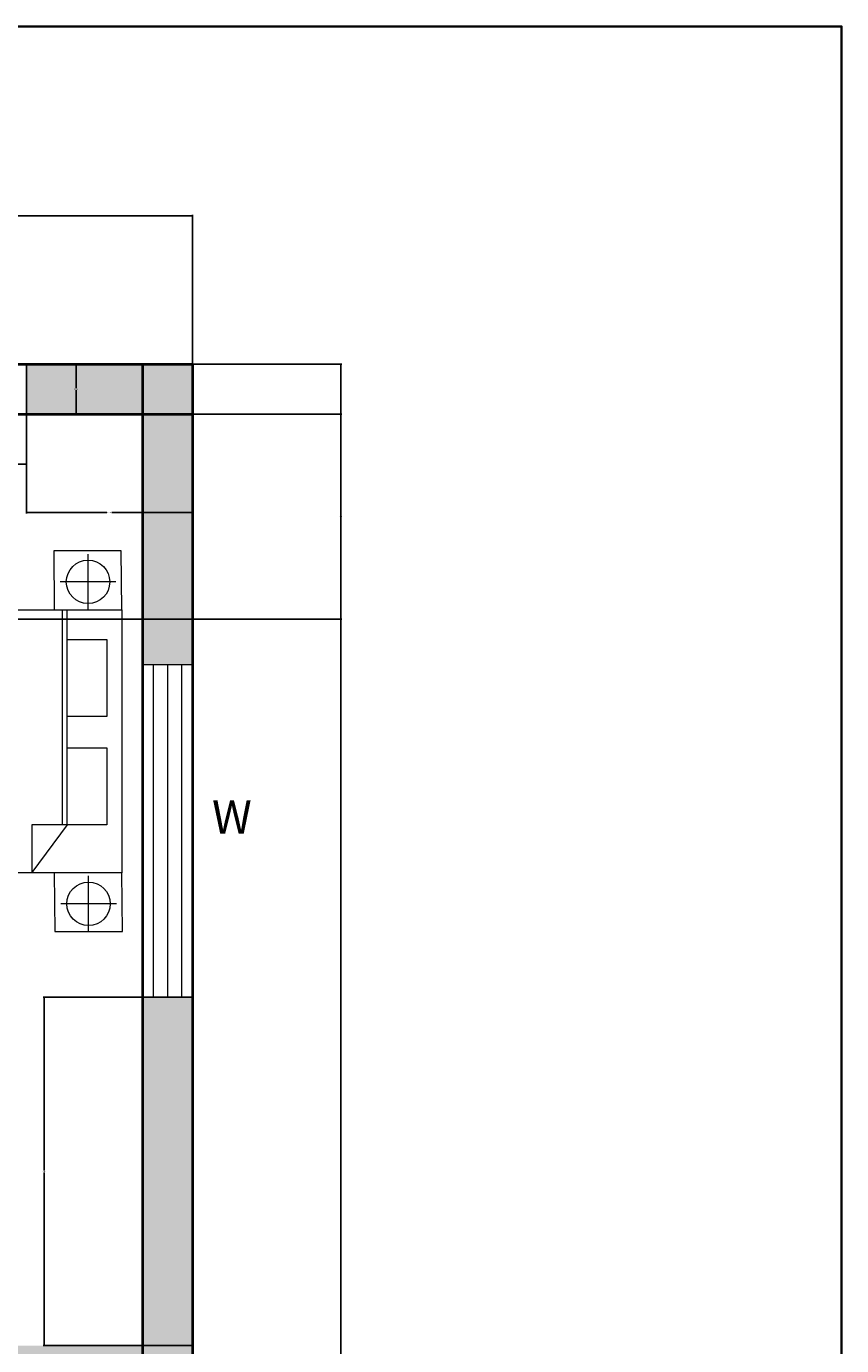
# Model space of a CAD drawing. Units: inches. Extents: x 25176543 to 25177243, y 80295576 to 80296086.
# Tile 11 of 11: x 25177096 to 25177243, y 80295848 to 80296086. Entities that reach past the tile are written whole.
import ezdxf

# ---------------------------------------------------------------- set-up
doc = ezdxf.new("R2010")
doc.units = ezdxf.units.IN
doc.header["$MEASUREMENT"] = 0
for name, color, linetype, lineweight in [('A-ANNO-DIMS', 2, 'Continuous', 18), ('A-ANNO-IDEN', 7, 'Continuous', 18), ('A-ANNO-TTLB', 7, 'Continuous', 35), ('A-COLS-PATT', 251, 'Continuous', 13), ('A-GLAZ', 4, 'Continuous', 18), ('A-WALL', 7, 'Continuous', 40), ('A-WALL-PATT', 146, 'Continuous', 13), ('furniture', 31, 'Continuous', 13)]:
    doc.layers.add(name, color=color, linetype=linetype, lineweight=lineweight)
doc.styles.get("Standard").update_dxf_attribs({"font": 'arial.ttf'})
doc.dimstyles.get("Standard").update_dxf_attribs({"dimtxt": 0.18, "dimasz": 0.18, "dimexe": 0.18, "dimexo": 0.0625, "dimgap": 0.09, "dimtad": 0, "dimtih": 1, "dimtoh": 1, "dimdec": 4, "dimzin": 0, "dimdsep": 46, "dimtxsty": 'Standard', "dimcen": 0.09, "dimadec": 0, "dimazin": 0, "dimtfac": 1, "dimtdec": 4, "dimtofl": 0, "dimtmove": 0, "dimatfit": 3, "dimfxl": 1, "dimtolj": 1, "dimtzin": 0, "dimarcsym": 0})

# ---------------------------------------------------------------- blocks, each defined once
blk = doc.blocks.new('BED-DOUBLE-WITH-NIGHTSTANDS')
for p, q in [((5.6, 61.62), (5.6, 51.56)), ((63.65, 61.72), (63.65, 51.66)), ((10.63, 56.59), (0.57, 56.59)), ((68.68, 56.69), (58.62, 56.69)), ((49.39, 52.82), (10.63, 52.82)), ((49.39, 52.82), (58, 46.47)), ((49.44, 52.82), (49.44, 46.47)), ((49.44, 52), (10.63, 52)), ((49.44, 46.47), (58, 46.47)), ((58.05, 34.96), (10.63, 34.96)), ((4.35, 0), (4.35, 26.37)), ((4.35, 26.37), (10.65, 26.37)), ((58.05, 26.37), (67.59, 26.37)), ((67.59, 26.37), (67.59, 0)), ((67.59, 0), (4.35, 0))]:
    blk.add_line(p, q)
for points in [[(0, 50.39), (10.63, 50.5), (10.63, 62.68), (0, 62.58)], [(58.05, 62.68), (58.05, 11.37), (10.63, 11.37), (10.63, 62.68)], [(58.05, 50.5), (68.68, 50.6), (68.68, 62.78), (58.05, 62.68)], [(29.88, 59.98), (29.88, 52.82), (15.98, 52.82), (15.98, 59.98)], [(49.44, 59.98), (49.44, 52.82), (35.55, 52.82), (35.55, 59.98)]]:
    blk.add_lwpolyline(points, close=True)
for centre in [(5.6, 56.59), (63.65, 56.69)]:
    blk.add_circle(centre, 3.92)
for points, knots in [([(3.23, 25.84), (3.32, 25.96), (3.52, 26.2), (3.86, 25.96), (4.14, 25.78), (4.29, 25.89), (4.35, 25.94)], [0, 0, 0, 0, 0.400747, 0.791423, 1.067667, 1.29709, 1.29709, 1.29709, 1.29709]), ([(3.23, 25.06), (3.32, 25.18), (3.52, 25.42), (3.86, 25.18), (4.14, 25.01), (4.29, 25.11), (4.35, 25.16)], [0, 0, 0, 0, 0.400747, 0.791423, 1.067667, 1.29709, 1.29709, 1.29709, 1.29709]), ([(3.23, 24.24), (3.32, 24.36), (3.52, 24.6), (3.86, 24.36), (4.14, 24.19), (4.29, 24.3), (4.35, 24.34)], [0, 0, 0, 0, 0.400747, 0.791423, 1.067667, 1.29709, 1.29709, 1.29709, 1.29709]), ([(68.71, 25.84), (68.61, 25.96), (68.42, 26.2), (68.08, 25.96), (67.8, 25.78), (67.65, 25.89), (67.58, 25.94)], [0, 0, 0, 0, 0.400747, 0.791423, 1.067667, 1.29709, 1.29709, 1.29709, 1.29709]), ([(68.71, 25.06), (68.61, 25.18), (68.42, 25.42), (68.08, 25.18), (67.8, 25.01), (67.65, 25.11), (67.58, 25.16)], [0, 0, 0, 0, 0.400747, 0.791423, 1.067667, 1.29709, 1.29709, 1.29709, 1.29709]), ([(68.71, 24.24), (68.61, 24.36), (68.42, 24.6), (68.08, 24.36), (67.8, 24.19), (67.65, 24.3), (67.58, 24.34)], [0, 0, 0, 0, 0.400747, 0.791423, 1.067667, 1.29709, 1.29709, 1.29709, 1.29709]), ([(3.23, 23.51), (3.32, 23.63), (3.52, 23.87), (3.86, 23.63), (4.14, 23.46), (4.29, 23.57), (4.35, 23.62)], [0, 0, 0, 0, 0.400747, 0.791423, 1.067667, 1.29709, 1.29709, 1.29709, 1.29709]), ([(3.23, 22.63), (3.32, 22.75), (3.52, 22.99), (3.86, 22.75), (4.14, 22.58), (4.29, 22.69), (4.35, 22.73)], [0, 0, 0, 0, 0.400747, 0.791423, 1.067667, 1.29709, 1.29709, 1.29709, 1.29709]), ([(3.23, 21.88), (3.32, 22), (3.52, 22.24), (3.86, 22), (4.14, 21.83), (4.29, 21.93), (4.35, 21.98)], [0, 0, 0, 0, 0.400747, 0.791423, 1.067667, 1.29709, 1.29709, 1.29709, 1.29709]), ([(3.23, 21.15), (3.32, 21.27), (3.52, 21.51), (3.86, 21.27), (4.14, 21.1), (4.29, 21.21), (4.35, 21.25)], [0, 0, 0, 0, 0.400747, 0.791423, 1.067667, 1.29709, 1.29709, 1.29709, 1.29709]), ([(68.71, 23.51), (68.61, 23.63), (68.42, 23.87), (68.08, 23.63), (67.8, 23.46), (67.65, 23.57), (67.58, 23.62)], [0, 0, 0, 0, 0.400747, 0.791423, 1.067667, 1.29709, 1.29709, 1.29709, 1.29709]), ([(68.71, 22.63), (68.61, 22.75), (68.42, 22.99), (68.08, 22.75), (67.8, 22.58), (67.65, 22.69), (67.58, 22.73)], [0, 0, 0, 0, 0.400747, 0.791423, 1.067667, 1.29709, 1.29709, 1.29709, 1.29709]), ([(68.71, 21.88), (68.61, 22), (68.42, 22.24), (68.08, 22), (67.8, 21.83), (67.65, 21.93), (67.58, 21.98)], [0, 0, 0, 0, 0.400747, 0.791423, 1.067667, 1.29709, 1.29709, 1.29709, 1.29709]), ([(68.71, 21.15), (68.61, 21.27), (68.42, 21.51), (68.08, 21.27), (67.8, 21.1), (67.65, 21.21), (67.58, 21.25)], [0, 0, 0, 0, 0.400747, 0.791423, 1.067667, 1.29709, 1.29709, 1.29709, 1.29709]), ([(3.23, 20.27), (3.32, 20.39), (3.52, 20.63), (3.86, 20.39), (4.14, 20.22), (4.29, 20.32), (4.35, 20.37)], [0, 0, 0, 0, 0.400747, 0.791423, 1.067667, 1.29709, 1.29709, 1.29709, 1.29709]), ([(3.23, 19.23), (3.32, 19.35), (3.52, 19.59), (3.86, 19.35), (4.14, 19.18), (4.29, 19.29), (4.35, 19.33)], [0, 0, 0, 0, 0.400747, 0.791423, 1.067667, 1.29709, 1.29709, 1.29709, 1.29709]), ([(68.71, 20.27), (68.61, 20.39), (68.42, 20.63), (68.08, 20.39), (67.8, 20.22), (67.65, 20.32), (67.58, 20.37)], [0, 0, 0, 0, 0.400747, 0.791423, 1.067667, 1.29709, 1.29709, 1.29709, 1.29709]), ([(68.71, 19.23), (68.61, 19.35), (68.42, 19.59), (68.08, 19.35), (67.8, 19.18), (67.65, 19.29), (67.58, 19.33)], [0, 0, 0, 0, 0.400747, 0.791423, 1.067667, 1.29709, 1.29709, 1.29709, 1.29709]), ([(3.23, 18.35), (3.32, 18.47), (3.52, 18.71), (3.86, 18.47), (4.14, 18.3), (4.29, 18.4), (4.35, 18.45)], [0, 0, 0, 0, 0.400747, 0.791423, 1.067667, 1.29709, 1.29709, 1.29709, 1.29709]), ([(3.23, 17.53), (3.32, 17.65), (3.52, 17.89), (3.86, 17.65), (4.14, 17.48), (4.29, 17.59), (4.35, 17.64)], [0, 0, 0, 0, 0.400747, 0.791423, 1.067667, 1.29709, 1.29709, 1.29709, 1.29709]), ([(3.23, 16.76), (3.32, 16.88), (3.52, 17.12), (3.86, 16.88), (4.14, 16.7), (4.29, 16.81), (4.35, 16.86)], [0, 0, 0, 0, 0.400747, 0.791423, 1.067667, 1.29709, 1.29709, 1.29709, 1.29709]), ([(68.71, 18.35), (68.61, 18.47), (68.42, 18.71), (68.08, 18.47), (67.8, 18.3), (67.65, 18.4), (67.58, 18.45)], [0, 0, 0, 0, 0.400747, 0.791423, 1.067667, 1.29709, 1.29709, 1.29709, 1.29709]), ([(68.71, 17.53), (68.61, 17.65), (68.42, 17.89), (68.08, 17.65), (67.8, 17.48), (67.65, 17.59), (67.58, 17.64)], [0, 0, 0, 0, 0.400747, 0.791423, 1.067667, 1.29709, 1.29709, 1.29709, 1.29709]), ([(68.71, 16.76), (68.61, 16.88), (68.42, 17.12), (68.08, 16.88), (67.8, 16.7), (67.65, 16.81), (67.58, 16.86)], [0, 0, 0, 0, 0.400747, 0.791423, 1.067667, 1.29709, 1.29709, 1.29709, 1.29709]), ([(3.23, 15.94), (3.32, 16.06), (3.52, 16.3), (3.86, 16.06), (4.14, 15.89), (4.29, 16), (4.35, 16.04)], [0, 0, 0, 0, 0.400747, 0.791423, 1.067667, 1.29709, 1.29709, 1.29709, 1.29709]), ([(3.23, 15.21), (3.32, 15.33), (3.52, 15.57), (3.86, 15.33), (4.14, 15.16), (4.29, 15.27), (4.35, 15.32)], [0, 0, 0, 0, 0.400747, 0.791423, 1.067667, 1.29709, 1.29709, 1.29709, 1.29709]), ([(3.23, 14.33), (3.32, 14.45), (3.52, 14.69), (3.86, 14.45), (4.14, 14.28), (4.29, 14.38), (4.35, 14.43)], [0, 0, 0, 0, 0.400747, 0.791423, 1.067667, 1.29709, 1.29709, 1.29709, 1.29709]), ([(68.71, 15.94), (68.61, 16.06), (68.42, 16.3), (68.08, 16.06), (67.8, 15.89), (67.65, 16), (67.58, 16.04)], [0, 0, 0, 0, 0.400747, 0.791423, 1.067667, 1.29709, 1.29709, 1.29709, 1.29709]), ([(68.71, 15.21), (68.61, 15.33), (68.42, 15.57), (68.08, 15.33), (67.8, 15.16), (67.65, 15.27), (67.58, 15.32)], [0, 0, 0, 0, 0.400747, 0.791423, 1.067667, 1.29709, 1.29709, 1.29709, 1.29709]), ([(68.71, 14.33), (68.61, 14.45), (68.42, 14.69), (68.08, 14.45), (67.8, 14.28), (67.65, 14.38), (67.58, 14.43)], [0, 0, 0, 0, 0.400747, 0.791423, 1.067667, 1.29709, 1.29709, 1.29709, 1.29709]), ([(3.23, 13.58), (3.32, 13.7), (3.52, 13.94), (3.86, 13.7), (4.14, 13.53), (4.29, 13.63), (4.35, 13.68)], [0, 0, 0, 0, 0.400747, 0.791423, 1.067667, 1.29709, 1.29709, 1.29709, 1.29709]), ([(3.23, 12.85), (3.32, 12.97), (3.52, 13.21), (3.86, 12.97), (4.14, 12.8), (4.29, 12.9), (4.35, 12.95)], [0, 0, 0, 0, 0.400747, 0.791423, 1.067667, 1.29709, 1.29709, 1.29709, 1.29709]), ([(3.23, 11.97), (3.32, 12.09), (3.52, 12.33), (3.86, 12.09), (4.14, 11.92), (4.29, 12.02), (4.35, 12.07)], [0, 0, 0, 0, 0.400747, 0.791423, 1.067667, 1.29709, 1.29709, 1.29709, 1.29709]), ([(68.71, 13.58), (68.61, 13.7), (68.42, 13.94), (68.08, 13.7), (67.8, 13.53), (67.65, 13.63), (67.58, 13.68)], [0, 0, 0, 0, 0.400747, 0.791423, 1.067667, 1.29709, 1.29709, 1.29709, 1.29709]), ([(68.71, 12.85), (68.61, 12.97), (68.42, 13.21), (68.08, 12.97), (67.8, 12.8), (67.65, 12.9), (67.58, 12.95)], [0, 0, 0, 0, 0.400747, 0.791423, 1.067667, 1.29709, 1.29709, 1.29709, 1.29709]), ([(68.71, 11.97), (68.61, 12.09), (68.42, 12.33), (68.08, 12.09), (67.8, 11.92), (67.65, 12.02), (67.58, 12.07)], [0, 0, 0, 0, 0.400747, 0.791423, 1.067667, 1.29709, 1.29709, 1.29709, 1.29709]), ([(3.23, 10.93), (3.32, 11.05), (3.52, 11.29), (3.86, 11.05), (4.14, 10.88), (4.29, 10.99), (4.35, 11.03)], [0, 0, 0, 0, 0.400747, 0.791423, 1.067667, 1.29709, 1.29709, 1.29709, 1.29709]), ([(3.23, 10.05), (3.32, 10.17), (3.52, 10.41), (3.86, 10.17), (4.14, 10), (4.29, 10.1), (4.35, 10.15)], [0, 0, 0, 0, 0.400747, 0.791423, 1.067667, 1.29709, 1.29709, 1.29709, 1.29709]), ([(68.71, 10.93), (68.61, 11.05), (68.42, 11.29), (68.08, 11.05), (67.8, 10.88), (67.65, 10.99), (67.58, 11.03)], [0, 0, 0, 0, 0.400747, 0.791423, 1.067667, 1.29709, 1.29709, 1.29709, 1.29709]), ([(68.71, 10.05), (68.61, 10.17), (68.42, 10.41), (68.08, 10.17), (67.8, 10), (67.65, 10.1), (67.58, 10.15)], [0, 0, 0, 0, 0.400747, 0.791423, 1.067667, 1.29709, 1.29709, 1.29709, 1.29709]), ([(3.23, 9.23), (3.32, 9.35), (3.52, 9.59), (3.86, 9.35), (4.14, 9.18), (4.29, 9.29), (4.35, 9.34)], [0, 0, 0, 0, 0.400747, 0.791423, 1.067667, 1.29709, 1.29709, 1.29709, 1.29709]), ([(3.23, 8.54), (3.32, 8.66), (3.52, 8.9), (3.86, 8.66), (4.14, 8.49), (4.29, 8.6), (4.35, 8.65)], [0, 0, 0, 0, 0.400747, 0.791423, 1.067667, 1.29709, 1.29709, 1.29709, 1.29709]), ([(3.23, 7.73), (3.32, 7.85), (3.52, 8.09), (3.86, 7.85), (4.14, 7.68), (4.29, 7.78), (4.35, 7.83)], [0, 0, 0, 0, 0.400747, 0.791423, 1.067667, 1.29709, 1.29709, 1.29709, 1.29709]), ([(3.23, 7), (3.32, 7.12), (3.52, 7.36), (3.86, 7.12), (4.14, 6.95), (4.29, 7.05), (4.35, 7.1)], [0, 0, 0, 0, 0.400747, 0.791423, 1.067667, 1.29709, 1.29709, 1.29709, 1.29709]), ([(68.71, 9.23), (68.61, 9.35), (68.42, 9.59), (68.08, 9.35), (67.8, 9.18), (67.65, 9.29), (67.58, 9.34)], [0, 0, 0, 0, 0.400747, 0.791423, 1.067667, 1.29709, 1.29709, 1.29709, 1.29709]), ([(68.71, 8.54), (68.61, 8.66), (68.42, 8.9), (68.08, 8.66), (67.8, 8.49), (67.65, 8.6), (67.58, 8.65)], [0, 0, 0, 0, 0.400747, 0.791423, 1.067667, 1.29709, 1.29709, 1.29709, 1.29709]), ([(68.71, 7.73), (68.61, 7.85), (68.42, 8.09), (68.08, 7.85), (67.8, 7.68), (67.65, 7.78), (67.58, 7.83)], [0, 0, 0, 0, 0.400747, 0.791423, 1.067667, 1.29709, 1.29709, 1.29709, 1.29709]), ([(68.71, 7), (68.61, 7.12), (68.42, 7.36), (68.08, 7.12), (67.8, 6.95), (67.65, 7.05), (67.58, 7.1)], [0, 0, 0, 0, 0.400747, 0.791423, 1.067667, 1.29709, 1.29709, 1.29709, 1.29709]), ([(3.23, 6.12), (3.32, 6.24), (3.52, 6.48), (3.86, 6.24), (4.14, 6.07), (4.29, 6.17), (4.35, 6.22)], [0, 0, 0, 0, 0.400747, 0.791423, 1.067667, 1.29709, 1.29709, 1.29709, 1.29709]), ([(3.23, 5.36), (3.32, 5.49), (3.52, 5.73), (3.86, 5.49), (4.14, 5.31), (4.29, 5.42), (4.35, 5.47)], [0, 0, 0, 0, 0.400747, 0.791423, 1.067667, 1.29709, 1.29709, 1.29709, 1.29709]), ([(3.23, 4.64), (3.32, 4.76), (3.52, 5), (3.86, 4.76), (4.14, 4.59), (4.29, 4.69), (4.35, 4.74)], [0, 0, 0, 0, 0.400747, 0.791423, 1.067667, 1.29709, 1.29709, 1.29709, 1.29709]), ([(68.71, 6.12), (68.61, 6.24), (68.42, 6.48), (68.08, 6.24), (67.8, 6.07), (67.65, 6.17), (67.58, 6.22)], [0, 0, 0, 0, 0.400747, 0.791423, 1.067667, 1.29709, 1.29709, 1.29709, 1.29709]), ([(68.71, 5.36), (68.61, 5.49), (68.42, 5.73), (68.08, 5.49), (67.8, 5.31), (67.65, 5.42), (67.58, 5.47)], [0, 0, 0, 0, 0.400747, 0.791423, 1.067667, 1.29709, 1.29709, 1.29709, 1.29709]), ([(68.71, 4.64), (68.61, 4.76), (68.42, 5), (68.08, 4.76), (67.8, 4.59), (67.66, 4.69), (67.59, 4.73)], [0, 0, 0, 0, 0.400747, 0.791423, 1.067667, 1.283686, 1.283686, 1.283686, 1.283686]), ([(3.23, 3.75), (3.32, 3.88), (3.52, 4.12), (3.86, 3.88), (4.14, 3.7), (4.29, 3.81), (4.35, 3.86)], [0, 0, 0, 0, 0.400747, 0.791423, 1.067667, 1.29709, 1.29709, 1.29709, 1.29709]), ([(3.23, 3.33), (3.32, 3.45), (3.52, 3.7), (3.86, 3.44), (4.14, 3.27), (4.29, 3.38), (4.35, 3.43)], [0, 0, 0, 0, 0.407265, 0.802015, 1.07826, 1.307683, 1.307683, 1.307683, 1.307683]), ([(3.23, 2.76), (3.32, 2.88), (3.52, 3.12), (3.86, 2.88), (4.14, 2.71), (4.29, 2.81), (4.35, 2.86)], [0, 0, 0, 0, 0.400747, 0.791423, 1.067667, 1.29709, 1.29709, 1.29709, 1.29709]), ([(3.23, 2.18), (3.32, 2.31), (3.52, 2.55), (3.86, 2.31), (4.14, 2.13), (4.29, 2.24), (4.35, 2.29)], [0, 0, 0, 0, 0.400747, 0.791423, 1.067667, 1.29709, 1.29709, 1.29709, 1.29709]), ([(68.71, 3.75), (68.61, 3.88), (68.42, 4.11), (68.08, 3.88), (67.8, 3.7), (67.66, 3.81), (67.59, 3.85)], [0, 0, 0, 0, 0.400747, 0.791423, 1.067667, 1.283686, 1.283686, 1.283686, 1.283686]), ([(68.71, 3.33), (68.61, 3.45), (68.42, 3.69), (68.08, 3.45), (67.8, 3.27), (67.66, 3.38), (67.59, 3.42)], [0, 0, 0, 0, 0.402903, 0.794912, 1.071156, 1.287177, 1.287177, 1.287177, 1.287177]), ([(68.71, 2.73), (68.61, 2.85), (68.42, 3.09), (68.08, 2.85), (67.8, 2.68), (67.66, 2.78), (67.59, 2.82)], [0, 0, 0, 0, 0.400747, 0.791423, 1.067667, 1.283686, 1.283686, 1.283686, 1.283686]), ([(68.71, 2.16), (68.61, 2.28), (68.42, 2.52), (68.08, 2.28), (67.8, 2.11), (67.66, 2.21), (67.59, 2.25)], [0, 0, 0, 0, 0.400747, 0.791423, 1.067667, 1.283686, 1.283686, 1.283686, 1.283686]), ([(3.23, 1.88), (3.32, 2), (3.52, 2.24), (3.86, 2), (4.14, 1.82), (4.29, 1.93), (4.35, 1.98)], [0, 0, 0, 0, 0.400747, 0.791423, 1.067667, 1.29709, 1.29709, 1.29709, 1.29709]), ([(3.23, 1.46), (3.32, 1.58), (3.52, 1.82), (3.86, 1.58), (4.14, 1.41), (4.29, 1.51), (4.35, 1.56)], [0, 0, 0, 0, 0.400747, 0.791423, 1.067667, 1.29709, 1.29709, 1.29709, 1.29709]), ([(3.23, 1.06), (3.32, 1.18), (3.52, 1.42), (3.86, 1.18), (4.14, 1.01), (4.29, 1.11), (4.35, 1.16)], [0, 0, 0, 0, 0.400747, 0.791423, 1.067667, 1.29709, 1.29709, 1.29709, 1.29709]), ([(3.23, 0.57), (3.32, 0.7), (3.52, 0.94), (3.86, 0.7), (4.14, 0.52), (4.29, 0.63), (4.35, 0.68)], [0, 0, 0, 0, 0.400747, 0.791423, 1.067667, 1.29709, 1.29709, 1.29709, 1.29709]), ([(3.23, 0.07), (3.32, 0.19), (3.52, 0.43), (3.86, 0.19), (4.14, 0.02), (4.29, 0.13), (4.35, 0.18)], [0, 0, 0, 0, 0.400747, 0.791423, 1.067667, 1.29709, 1.29709, 1.29709, 1.29709]), ([(68.71, 1.43), (68.61, 1.55), (68.42, 1.79), (68.08, 1.55), (67.8, 1.38), (67.65, 1.48), (67.58, 1.53)], [0, 0, 0, 0, 0.400747, 0.791423, 1.067667, 1.29709, 1.29709, 1.29709, 1.29709]), ([(68.71, 1.03), (68.61, 1.15), (68.42, 1.39), (68.08, 1.15), (67.8, 0.98), (67.65, 1.09), (67.58, 1.13)], [0, 0, 0, 0, 0.400747, 0.791423, 1.067667, 1.29709, 1.29709, 1.29709, 1.29709]), ([(68.71, 0.55), (68.61, 0.67), (68.42, 0.91), (68.08, 0.67), (67.8, 0.49), (67.65, 0.6), (67.58, 0.65)], [0, 0, 0, 0, 0.400747, 0.791423, 1.067667, 1.29709, 1.29709, 1.29709, 1.29709]), ([(68.71, 0.07), (68.61, 0.19), (68.42, 0.43), (68.08, 0.19), (67.8, 0.02), (67.65, 0.13), (67.58, 0.18)], [0, 0, 0, 0, 0.400747, 0.791423, 1.067667, 1.29709, 1.29709, 1.29709, 1.29709]), ([(68.71, 1.85), (68.61, 1.97), (68.42, 2.21), (68.08, 1.97), (67.8, 1.8), (67.66, 1.9), (67.59, 1.94)], [0, 0, 0, 0, 0.400747, 0.791423, 1.067667, 1.283686, 1.283686, 1.283686, 1.283686])]:
    blk.add_open_spline(points, degree=3, knots=knots)
blk = doc.blocks.new('WIN-60IN')
for p, q in [((0, 9), (0, 0)), ((60, 9), (0, 9)), ((0, 9), (0, 4.5)), ((60, 0), (60, 9)), ((60, 7), (0, 7)), ((0, 4.5), (60, 4.5)), ((0, 2), (60, 2)), ((0, 0), (60, 0))]:
    blk.add_line(p, q)
blk = doc.blocks.new('*D20')
at = {"layer": 'A-ANNO-DIMS', "color": 0, "lineweight": -2, "transparency": 16777216}
for p, q in [((25177035.84, 80296016.24), (25177035.84, 80296007.12)), ((25177095.84, 80296016.24), (25177095.84, 80296007.12)), ((25177036.02, 80296007.3), (25177064.73, 80296007.3)), ((25177095.66, 80296007.3), (25177066.96, 80296007.3))]:
    blk.add_line(p, q, dxfattribs=at)
at = {"layer": 'A-ANNO-DIMS', "color": 0, "transparency": 16777216}
for points in [[(25177036.02, 80296007.33), (25177036.02, 80296007.27), (25177035.84, 80296007.3)], [(25177095.66, 80296007.33), (25177095.66, 80296007.27), (25177095.84, 80296007.3)]]:
    blk.add_solid(points, dxfattribs=at)
at = {"layer": 'Defpoints', "color": 0, "transparency": 16777216}
for p in [(25177035.84, 80296016.3), (25177095.84, 80296016.3), (25177095.84, 80296007.3)]:
    blk.add_point(p, dxfattribs=at)
at = {"layer": 'A-ANNO-DIMS', "color": 0, "transparency": 16777216, "insert": (25177065.84, 80296007.3), "char_height": 0.18, "attachment_point": 5}
blk.add_mtext('\\A1;WINDOW 60 TYP.', dxfattribs=at)
blk = doc.blocks.new('*D21')
at = {"layer": 'A-ANNO-DIMS', "color": 0, "lineweight": -2, "transparency": 16777216}
for p, q in [((25177095.91, 80296025.3), (25177105.02, 80296025.3)), ((25177104.84, 80296025.12), (25177104.84, 80296020.98)), ((25177104.84, 80296016.48), (25177104.84, 80296020.62)), ((25177095.91, 80296016.3), (25177105.02, 80296016.3))]:
    blk.add_line(p, q, dxfattribs=at)
at = {"layer": 'A-ANNO-DIMS', "color": 0, "transparency": 16777216}
for points in [[(25177104.81, 80296025.12), (25177104.87, 80296025.12), (25177104.84, 80296025.3)], [(25177104.81, 80296016.48), (25177104.87, 80296016.48), (25177104.84, 80296016.3)]]:
    blk.add_solid(points, dxfattribs=at)
at = {"layer": 'Defpoints', "color": 0, "transparency": 16777216}
for p in [(25177095.84, 80296025.3), (25177104.84, 80296025.3), (25177095.84, 80296016.3)]:
    blk.add_point(p, dxfattribs=at)
at = {"layer": 'A-ANNO-DIMS', "color": 0, "transparency": 16777216, "insert": (25177104.84, 80296020.8), "char_height": 0.18, "attachment_point": 5}
blk.add_mtext('\\A1;9 TYP.', dxfattribs=at)
blk = doc.blocks.new('*D48')
at = {"layer": 'A-ANNO-DIMS', "color": 0, "lineweight": -2, "transparency": 16777216}
for p, q in [((25176625.3, 80295890.36), (25176625.3, 80296052.23)), ((25176625.48, 80296052.05), (25176875.16, 80296052.05)), ((25177125.62, 80296052.05), (25176875.95, 80296052.05)), ((25177125.8, 80296025.36), (25177125.8, 80296052.23))]:
    blk.add_line(p, q, dxfattribs=at)
at = {"layer": 'A-ANNO-DIMS', "color": 0, "transparency": 16777216}
for points in [[(25176625.48, 80296052.08), (25176625.48, 80296052.02), (25176625.3, 80296052.05)], [(25177125.62, 80296052.08), (25177125.62, 80296052.02), (25177125.8, 80296052.05)]]:
    blk.add_solid(points, dxfattribs=at)
at = {"layer": 'Defpoints', "color": 0, "transparency": 16777216}
for p in [(25177125.8, 80296052.05), (25177125.8, 80296025.3), (25176625.3, 80295890.3)]:
    blk.add_point(p, dxfattribs=at)
at = {"layer": 'A-ANNO-DIMS', "color": 0, "transparency": 16777216, "insert": (25176875.55, 80296052.05), "char_height": 0.18, "attachment_point": 5}
blk.add_mtext('\\A1;500.5', dxfattribs=at)
blk = doc.blocks.new('*D49')
at = {"layer": 'A-ANNO-DIMS', "color": 0, "lineweight": -2, "transparency": 16777216}
for p, q in [((25177125.86, 80296025.3), (25177152.73, 80296025.3)), ((25177152.55, 80296025.12), (25177152.55, 80295846.73)), ((25177152.55, 80295667.98), (25177152.55, 80295846.37)), ((25177125.86, 80295667.8), (25177152.73, 80295667.8))]:
    blk.add_line(p, q, dxfattribs=at)
at = {"layer": 'A-ANNO-DIMS', "color": 0, "transparency": 16777216}
for points in [[(25177152.52, 80296025.12), (25177152.58, 80296025.12), (25177152.55, 80296025.3)], [(25177152.52, 80295667.98), (25177152.58, 80295667.98), (25177152.55, 80295667.8)]]:
    blk.add_solid(points, dxfattribs=at)
at = {"layer": 'Defpoints', "color": 0, "transparency": 16777216}
for p in [(25177125.8, 80296025.3), (25177152.55, 80296025.3), (25177125.8, 80295667.8)]:
    blk.add_point(p, dxfattribs=at)
at = {"layer": 'A-ANNO-DIMS', "color": 0, "transparency": 16777216, "insert": (25177152.55, 80295846.55), "char_height": 0.18, "attachment_point": 5}
blk.add_mtext('\\A1;357.5', dxfattribs=at)
blk = doc.blocks.new('*D61')
at = {"layer": 'A-ANNO-DIMS', "color": 0, "lineweight": -2, "transparency": 16777216}
for p, q in [((25177125.74, 80295911.13), (25177098.87, 80295911.13)), ((25177099.05, 80295910.95), (25177099.05, 80295879.9)), ((25177099.05, 80295848.48), (25177099.05, 80295879.54)), ((25177125.74, 80295848.3), (25177098.87, 80295848.3))]:
    blk.add_line(p, q, dxfattribs=at)
at = {"layer": 'A-ANNO-DIMS', "color": 0, "transparency": 16777216}
for points in [[(25177099.02, 80295910.95), (25177099.08, 80295910.95), (25177099.05, 80295911.13)], [(25177099.02, 80295848.48), (25177099.08, 80295848.48), (25177099.05, 80295848.3)]]:
    blk.add_solid(points, dxfattribs=at)
at = {"layer": 'Defpoints', "color": 0, "transparency": 16777216}
for p in [(25177099.05, 80295911.13), (25177125.8, 80295911.13), (25177125.8, 80295848.3)]:
    blk.add_point(p, dxfattribs=at)
at = {"layer": 'A-ANNO-DIMS', "color": 0, "transparency": 16777216, "insert": (25177099.05, 80295879.72), "char_height": 0.18, "attachment_point": 5}
blk.add_mtext('\\A1;62.83', dxfattribs=at)
blk = doc.blocks.new('*D64')
at = {"layer": 'A-ANNO-DIMS', "color": 0, "lineweight": -2, "transparency": 16777216}
for p, q in [((25177095.84, 80296025.24), (25177095.84, 80295998.37)), ((25177125.8, 80296025.24), (25177125.8, 80295998.37)), ((25177096.02, 80295998.55), (25177110.36, 80295998.55)), ((25177125.62, 80295998.55), (25177111.29, 80295998.55))]:
    blk.add_line(p, q, dxfattribs=at)
at = {"layer": 'A-ANNO-DIMS', "color": 0, "transparency": 16777216}
for points in [[(25177096.02, 80295998.58), (25177096.02, 80295998.52), (25177095.84, 80295998.55)], [(25177125.62, 80295998.58), (25177125.62, 80295998.52), (25177125.8, 80295998.55)]]:
    blk.add_solid(points, dxfattribs=at)
at = {"layer": 'Defpoints', "color": 0, "transparency": 16777216}
for p in [(25177095.84, 80296025.3), (25177125.8, 80296025.3), (25177095.84, 80295998.55)]:
    blk.add_point(p, dxfattribs=at)
at = {"layer": 'A-ANNO-DIMS', "color": 0, "transparency": 16777216, "insert": (25177110.82, 80295998.55), "char_height": 0.18, "attachment_point": 5}
blk.add_mtext('\\A1;29.957', dxfattribs=at)
blk = doc.blocks.new('*D70')
at = {"layer": 'A-ANNO-DIMS', "color": 0, "lineweight": -2, "transparency": 16777216}
for p, q in [((25177004.36, 80296016.3), (25177152.73, 80296016.3)), ((25177152.55, 80296016.12), (25177152.55, 80295997.99)), ((25177152.55, 80295979.5), (25177152.55, 80295997.63)), ((25177004.36, 80295979.32), (25177152.73, 80295979.32))]:
    blk.add_line(p, q, dxfattribs=at)
at = {"layer": 'A-ANNO-DIMS', "color": 0, "transparency": 16777216}
for points in [[(25177152.52, 80296016.12), (25177152.58, 80296016.12), (25177152.55, 80296016.3)], [(25177152.52, 80295979.5), (25177152.58, 80295979.5), (25177152.55, 80295979.32)]]:
    blk.add_solid(points, dxfattribs=at)
at = {"layer": 'Defpoints', "color": 0, "transparency": 16777216}
for p in [(25177004.3, 80296016.3), (25177152.55, 80296016.3), (25177004.3, 80295979.32)]:
    blk.add_point(p, dxfattribs=at)
at = {"layer": 'A-ANNO-DIMS', "color": 0, "transparency": 16777216, "insert": (25177152.55, 80295997.81), "char_height": 0.18, "attachment_point": 5}
blk.add_mtext('\\A1;36.98', dxfattribs=at)

msp = doc.modelspace()

# ---------------------------------------------------------------- hatches: boundary and pattern name
at = {"layer": 'A-COLS-PATT'}
h = msp.add_hatch(color=256, dxfattribs=at)
h.dxf.hatch_style = 1
h.paths.add_polyline_path([(25176658.8016, 80296025.3022), (25176649.8016, 80296025.3022), (25176649.8016, 80296016.3022), (25176658.8016, 80296016.3022)])
h.paths.add_polyline_path([(25176819.3016, 80296025.3022), (25176810.3016, 80296025.3022), (25176810.3016, 80296016.3022), (25176819.3016, 80296016.3022)])
h.paths.add_polyline_path([(25176876.3016, 80296025.3022), (25176867.3016, 80296025.3022), (25176867.3016, 80296016.3022), (25176876.3016, 80296016.3022)])
h.paths.add_polyline_path([(25177013.3016, 80296025.3022), (25177004.3016, 80296025.3022), (25177004.3016, 80296016.3022), (25177013.3016, 80296016.3022)])
h.paths.add_polyline_path([(25176819.3016, 80295890.3022), (25176810.3016, 80295890.3022), (25176810.3016, 80295881.3022), (25176819.3016, 80295881.3022)])
h.paths.add_polyline_path([(25176658.8016, 80295890.3022), (25176649.8016, 80295890.3022), (25176649.8016, 80295881.3022), (25176658.8016, 80295881.3022)])
h.paths.add_polyline_path([(25177125.8016, 80296025.3022), (25177116.8016, 80296025.3022), (25177116.8016, 80296016.3022), (25177125.8016, 80296016.3022)])
h.paths.add_polyline_path([(25177125.8016, 80295848.3022), (25177116.8016, 80295848.3022), (25177116.8016, 80295839.3022), (25177125.8016, 80295839.3022)])
h.paths.add_polyline_path([(25177013.3016, 80295848.3022), (25177004.3016, 80295848.3022), (25177004.3016, 80295839.3022), (25177013.3016, 80295839.3022)])
h.paths.add_polyline_path([(25177125.8016, 80295676.8022), (25177116.8016, 80295676.8022), (25177116.8016, 80295667.8022), (25177125.8016, 80295667.8022)])
h.paths.add_polyline_path([(25177013.3016, 80295676.8022), (25177004.3016, 80295676.8022), (25177004.3016, 80295667.8022), (25177013.3016, 80295667.8022)])
h.paths.add_polyline_path([(25176842.3016, 80295676.8022), (25176833.3016, 80295676.8022), (25176833.3016, 80295667.8022), (25176842.3016, 80295667.8022)])
h.paths.add_polyline_path([(25176893.3016, 80295676.8022), (25176884.3016, 80295676.8022), (25176884.3016, 80295667.8022), (25176893.3016, 80295667.8022)])
h.paths.add_polyline_path([(25176842.3016, 80295807.3022), (25176833.3016, 80295807.3022), (25176833.3016, 80295798.3022), (25176842.3016, 80295798.3022)])
h.paths.add_polyline_path([(25176658.8016, 80295807.3022), (25176649.8016, 80295807.3022), (25176649.8016, 80295798.3022), (25176658.8016, 80295798.3022)])
h.paths.add_polyline_path([(25176658.8016, 80295676.8022), (25176649.8016, 80295676.8022), (25176649.8016, 80295667.8022), (25176658.8016, 80295667.8022)])
at = {"layer": 'A-WALL-PATT'}
h = msp.add_hatch(color=256, dxfattribs=at)
h.dxf.hatch_style = 1
h.paths.add_polyline_path([(25176695.189, 80296025.3022), (25176658.8016, 80296025.3022), (25176658.8016, 80296016.3022), (25176695.189, 80296016.3022)])
h.paths.add_polyline_path([(25176810.3016, 80296025.3022), (25176755.189, 80296025.3022), (25176755.189, 80296016.3022), (25176810.3016, 80296016.3022)])
h.paths.add_polyline_path([(25176819.3016, 80296016.3022), (25176814.8016, 80296016.3022), (25176814.8016, 80295965.3022), (25176819.3016, 80295965.3022)], flags=17)
h.paths.add_polyline_path([(25176828.0421, 80296025.3022), (25176819.3016, 80296025.3022), (25176819.3016, 80296016.3022), (25176828.0421, 80296016.3022)])
h.paths.add_polyline_path([(25176867.3016, 80296025.3022), (25176852.0421, 80296025.3022), (25176852.0421, 80296016.3022), (25176867.3016, 80296016.3022)])
h.paths.add_polyline_path([(25176885.1873, 80296025.3022), (25176876.3016, 80296025.3022), (25176876.3016, 80296016.3022), (25176885.1873, 80296016.3022)])
h.paths.add_polyline_path([(25176919.8016, 80296025.3022), (25176909.1873, 80296025.3022), (25176909.1873, 80296016.3022), (25176919.8016, 80296016.3022)])
h.paths.add_polyline_path([(25176924.3016, 80296016.3022), (25176919.8016, 80296016.3022), (25176919.8016, 80295890.3022), (25176904.8016, 80295890.3022), (25176904.8016, 80295885.8022), (25176967.3016, 80295885.8022), (25176967.3016, 80295890.3022), (25176924.3016, 80295890.3022)])
h.paths.add_polyline_path([(25176924.3016, 80296025.3022), (25176919.8016, 80296025.3022), (25176919.8016, 80296016.3022), (25176924.3016, 80296016.3022)])
h.paths.add_polyline_path([(25176938.7147, 80296025.3022), (25176924.3016, 80296025.3022), (25176924.3016, 80296016.3022), (25176938.7147, 80296016.3022)])
h.paths.add_polyline_path([(25176871.8016, 80296016.3022), (25176867.3016, 80296016.3022), (25176867.3016, 80295932.3022), (25176819.3016, 80295932.3022), (25176819.3016, 80295933.3022), (25176814.8016, 80295933.3022), (25176814.8016, 80295932.3022), (25176814.8016, 80295927.3022), (25176819.3016, 80295927.3022), (25176819.3016, 80295927.8022), (25176867.3016, 80295927.8022), (25176867.3016, 80295885.8022), (25176871.8016, 80295885.8022), (25176872.8016, 80295885.8022), (25176872.8016, 80295890.3022), (25176871.8016, 80295890.3022)])
h.paths.add_polyline_path([(25177004.3016, 80296025.3022), (25176986.7147, 80296025.3022), (25176986.7147, 80296016.3022), (25177004.3016, 80296016.3022)])
h.paths.add_polyline_path([(25177035.845, 80296025.3022), (25177013.3016, 80296025.3022), (25177013.3016, 80296016.3022), (25177035.845, 80296016.3022)])
h.paths.add_polyline_path([(25177008.8016, 80296016.3022), (25177004.3016, 80296016.3022), (25177004.3016, 80295890.3022), (25177003.3016, 80295890.3022), (25177003.3016, 80295885.8022), (25177004.3016, 80295885.8022), (25177004.3016, 80295885.3022), (25177008.8016, 80295885.3022)])
h.paths.add_polyline_path([(25177116.8016, 80296025.3022), (25177095.845, 80296025.3022), (25177095.845, 80296016.3022), (25177116.8016, 80296016.3022)])
h.paths.add_polyline_path([(25177125.8016, 80296016.3022), (25177116.8016, 80296016.3022), (25177116.8016, 80295971.1334), (25177121.3016, 80295971.1334), (25177125.8016, 80295971.1334)])
h.paths.add_polyline_path([(25177116.8016, 80295848.3022), (25177013.3016, 80295848.3022), (25177013.3016, 80295843.8022), (25177116.8016, 80295843.8022)])
h.paths.add_polyline_path([(25177125.8016, 80295911.1334), (25177116.8016, 80295911.1334), (25177116.8016, 80295848.3022), (25177125.8016, 80295848.3022)])
h.paths.add_polyline_path([(25177008.8016, 80295802.3022), (25177004.3016, 80295802.3022), (25177004.3016, 80295676.8022), (25177008.8016, 80295676.8022)])
h.paths.add_polyline_path([(25176658.8016, 80295705.5694), (25176649.8016, 80295705.5694), (25176649.8016, 80295676.8022), (25176658.8016, 80295676.8022)])
h.paths.add_polyline_path([(25176658.8016, 80295798.3022), (25176649.8016, 80295798.3022), (25176649.8016, 80295765.5694), (25176654.3016, 80295765.5694), (25176658.8016, 80295765.5694)])
h.paths.add_polyline_path([(25176833.3016, 80295807.3022), (25176658.8016, 80295807.3022), (25176658.8016, 80295802.8022), (25176833.3016, 80295802.8022)])
h.paths.add_polyline_path([(25176842.3016, 80295761.3022), (25176837.8016, 80295761.3022), (25176837.8016, 80295676.8022), (25176842.3016, 80295676.8022)])
h.paths.add_polyline_path([(25176649.8016, 80295807.3022), (25176629.8016, 80295807.3022), (25176629.8016, 80295885.8022), (25176649.8016, 80295885.8022), (25176649.8016, 80295890.3022), (25176625.3016, 80295890.3022), (25176625.3016, 80295802.8022), (25176649.8016, 80295802.8022)])
h.paths.add_polyline_path([(25176810.3016, 80295890.3022), (25176658.8016, 80295890.3022), (25176658.8016, 80295885.8022), (25176810.3016, 80295885.8022)])
h.paths.add_polyline_path([(25176658.8016, 80295922.9263), (25176649.8016, 80295922.9263), (25176649.8016, 80295890.3022), (25176658.8016, 80295890.3022)])
h.paths.add_polyline_path([(25176658.8016, 80296016.3022), (25176649.8016, 80296016.3022), (25176649.8016, 80295982.9263), (25176654.3016, 80295982.9263), (25176658.8016, 80295982.9263)])

# ---------------------------------------------------------------- linework, layer by layer
at = {"layer": 'A-ANNO-TTLB'}
msp.add_lwpolyline([(25176542.8973, 80296086.2335), (25177242.9194, 80296086.2335), (25177242.9194, 80295575.9501), (25176542.8973, 80295575.9501)], close=True, dxfattribs=at)
at = {"layer": 'A-WALL'}
for p, q in [((25176649.8016, 80296025.3022), (25177125.8016, 80296025.3022)), ((25177116.8016, 80296025.3022), (25177116.8016, 80295667.8022)), ((25177125.8016, 80296025.3022), (25177125.8016, 80295667.8022)), ((25176649.8016, 80296016.3022), (25177125.8016, 80296016.3022))]:
    msp.add_line(p, q, dxfattribs=at)

# ---------------------------------------------------------------- block references
at = {"layer": 'A-GLAZ', "extrusion": (0, 0, -1), "zscale": -1, "rotation": 270.0000000513552}
msp.add_blockref('WIN-60IN', (-25177125.8018, 80295971.1334), dxfattribs=at)
at = {"layer": 'furniture', "rotation": 269.9999999743436}
msp.add_blockref('BED-DOUBLE-WITH-NIGHTSTANDS', (25177050.3784, 80295991.6444), dxfattribs=at)

# ---------------------------------------------------------------- texts
at = {"layer": 'A-ANNO-IDEN', "insert": (25177129.3314, 80295946.6438), "char_height": 6, "attachment_point": 1}
msp.add_mtext_dynamic_manual_height_columns('W', width=24.139595, gutter_width=1, heights=[0], dxfattribs=at)

# ---------------------------------------------------------------- dimensions: what is measured, and where the dimension line sits
at = {"layer": 'A-ANNO-DIMS'}
dim = msp.add_linear_dim(base=(25177125.8016, 80296052.0522), p1=(25176625.3016, 80295890.3022), p2=(25177125.8016, 80296025.3022), dimstyle='Standard', override={"dimdec": 1, "dimlfac": 1, "dimrnd": 0, "dimzin": 0, "dimdsep": 46, "dimlunit": 2}, dxfattribs=at)
dim.commit()
dim.dimension.update_dxf_attribs({"geometry": '*D48', "text_midpoint": (25176875.5516, 80296052.0522)})
dim = msp.add_linear_dim(base=(25177104.845, 80296025.3022), p1=(25177095.845, 80296016.3022), p2=(25177095.845, 80296025.3022), angle=90, text='<> TYP.', dimstyle='Standard', override={"dimdec": 0, "dimlfac": 1, "dimrnd": 0, "dimzin": 0, "dimdsep": 46, "dimlunit": 2}, dxfattribs=at)
dim.commit()
dim.dimension.update_dxf_attribs({"geometry": '*D21', "text_midpoint": (25177104.845, 80296020.8022)})
for base, p1, p2, angle, override, picture, middle in [((25177095.845, 80295998.5522), (25177125.8016, 80296025.3022), (25177095.845, 80296025.3022), 180, {"dimdec": 3, "dimlfac": 1, "dimrnd": 0, "dimzin": 0, "dimdsep": 46, "dimlunit": 2}, '*D64', (25177110.8233, 80295998.5522)), ((25177152.5516, 80296025.3022), (25177125.8016, 80295667.8022), (25177125.8016, 80296025.3022), 90, {"dimdec": 1, "dimlfac": 1, "dimrnd": 0, "dimzin": 0, "dimdsep": 46, "dimlunit": 2}, '*D49', (25177152.5516, 80295846.5522)), ((25177152.5516, 80296016.3022), (25177004.3016, 80295979.3235), (25177004.3016, 80296016.3022), 90, {"dimdec": 2, "dimlfac": 1, "dimrnd": 0, "dimzin": 0, "dimdsep": 46, "dimlunit": 2}, '*D70', (25177152.5516, 80295997.8129)), ((25177099.0516, 80295911.1334), (25177125.8016, 80295848.3022), (25177125.8016, 80295911.1334), 90, {"dimdec": 2, "dimlfac": 1, "dimrnd": 0, "dimzin": 0, "dimdsep": 46, "dimlunit": 2}, '*D61', (25177099.0516, 80295879.7178))]:
    dim = msp.add_linear_dim(base=base, p1=p1, p2=p2, angle=angle, dimstyle='Standard', override=override, dxfattribs=at)
    dim.commit()
    dim.dimension.update_dxf_attribs({"geometry": picture, "text_midpoint": middle})
dim = msp.add_linear_dim(base=(25177095.845, 80296007.3022), p1=(25177035.845, 80296016.3022), p2=(25177095.845, 80296016.3022), text='WINDOW <> TYP.', dimstyle='Standard', override={"dimdec": 0, "dimlfac": 1, "dimrnd": 0, "dimzin": 0, "dimdsep": 46, "dimlunit": 2}, dxfattribs=at)
dim.commit()
dim.dimension.update_dxf_attribs({"geometry": '*D20', "text_midpoint": (25177065.845, 80296007.3022)})

doc.saveas('drawing.dxf')
